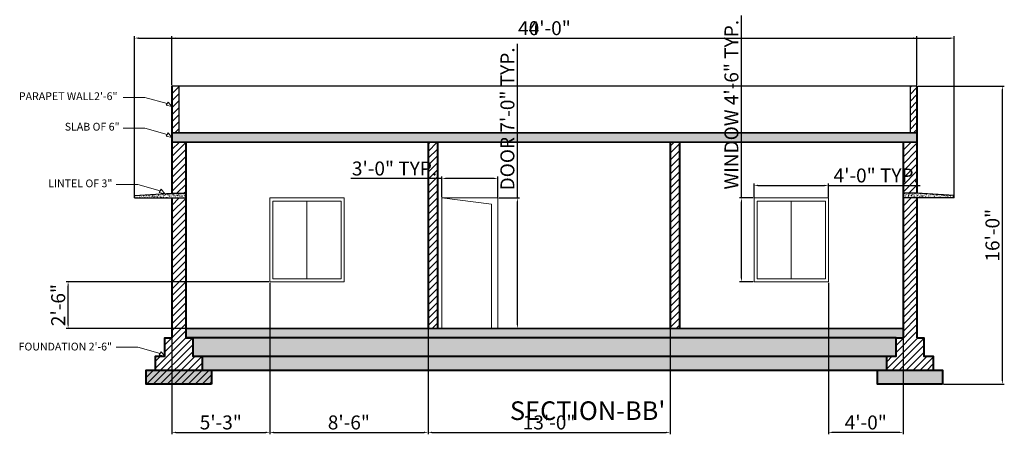
# Model space of a CAD drawing. Units: inches. Extents: x 2639 to 6021, y 292 to 2009.
# Tile 2 of 6: x 3381 to 4016, y 704 to 971. Entities that reach past the tile are written whole.
import ezdxf

# ---------------------------------------------------------------- set-up
doc = ezdxf.new("R2010")
doc.units = ezdxf.units.IN
for name, color, linetype, lineweight in [('A-ANNO-DIMS', 2, 'Continuous', 18), ('A-ANNO-TEXT', 7, 'Continuous', 18), ('A-DOOR', 3, 'Continuous', 20), ('A-GLAZ', 4, 'Continuous', 18), ('A-ROOF', 7, 'Continuous', 30), ('A-SECT', 7, 'Continuous', 40), ('A-SECT-PATT', 8, 'Continuous', 13), ('S-BEAM', 7, 'Continuous', 30), ('S-FNDN', 7, 'Continuous', 40), ('S-SLAB', 7, 'Continuous', 35)]:
    doc.layers.add(name, color=color, linetype=linetype, lineweight=lineweight)
doc.styles.get("Standard").update_dxf_attribs({"font": 'arial.ttf'})
doc.dimstyles.new('ISO-25', dxfattribs={"dimtxt": 9, "dimasz": 2.5, "dimexe": 1.25, "dimexo": 0.625, "dimtad": 1, "dimdec": 1, "dimlunit": 3, "dimtxsty": 'Standard', "dimcen": 2.5, "dimadec": 0, "dimazin": 0, "dimtfac": 1, "dimtdec": 1, "dimtmove": 0, "dimatfit": 3, "dimfxl": 1, "dimarcsym": 0})
pattern_1 = [(50, (-223.561, 0), (18.218467, -1.59391), [1.905, -20.955]), (355, (-223.561, 0), (-3.52434, 19.105685), [1.524, -16.76406]), (100.45144, (-222.043, -0.133), (14.694125, 17.511775), [1.619, -17.809024]), (46.1842, (-223.56, 5.08), (27.1079, -4.20423), [2.8575, -31.4325]), (96.63556, (-221.302, 4.73), (23.74041, 24.74261), [2.4285, -26.71356]), (351.18415, (-223.56, 5.08), (23.74041, 24.74261), [2.286, -25.14597]), (21, (-221.021, 3.81), (15.16144, -10.22652), [1.905, -20.955]), (326, (-221.021, 3.81), (6.1802, 18.4188), [1.524, -16.764]), (71.45144, (-219.758, 2.958), (21.34164, 8.19228), [1.619, -17.80899]), (37.5, (-223.561, 0), (0.30886, 8.455504), [0, -16.5608, 0, -17.018, 0, -16.8275]), (7.5, (-223.561, 0), (6.681966, 10.018057), [0, -9.7028, 0, -16.1798, 0, -6.4135]), (327.5, (-229.225, 0), (13.55906, -0.572874), [0, -6.35, 0, -19.812, 0, -26.289]), (317.5, (-231.765, 0), (14.812918, 2.54265), [0, -8.255, 0, -13.1572, 0, -18.669])]
pattern_2 = [(50, (-223.561, 0), (1.8218467, -0.15939086), [0.1905, -2.0955]), (355, (-223.561, 0), (-0.3524342, 1.91056845), [0.1524, -1.67640584]), (100.451445, (-223.4092, -0.0133), (1.4694125, 1.7511775), [0.1619001, -1.78090245]), (46.1842, (-223.561, 0.508), (2.7107904, -0.4204233), [0.28575, -3.14325]), (96.63556, (-223.3352, 0.473), (2.3740413, 2.4742612), [0.2428502, -2.671356]), (351.18415, (-223.561, 0.508), (2.3740413, 2.4742612), [0.2285997, -2.5145973]), (21, (-223.307, 0.381), (1.5161439, -1.022652), [0.1905, -2.0955]), (326, (-223.307, 0.381), (0.6180203, 1.8418797), [0.1524, -1.6764]), (71.451445, (-223.1807, 0.2958), (2.1341642, 0.8192277), [0.1619001, -1.7808994]), (37.5, (-223.56106, 0), (0.03088603, 0.84555039), [0, -1.65608, 0, -1.7018, 0, -1.68275]), (7.5, (-223.5611, 0), (0.66819663, 1.00180575), [0, -0.97028, 0, -1.61798, 0, -0.64135]), (327.5, (-224.1275, 0), (1.35590595, -0.05728744), [0, -0.635, 0, -1.9812, 0, -2.6289]), (317.5, (-224.3815, 0), (1.4812918, 0.2542649), [0, -0.8255, 0, -1.31572, 0, -1.8669])]

# ---------------------------------------------------------------- blocks, each defined once
blk = doc.blocks.new('DOOR-SECTION-36X84')
for p, q in [((0, 0), (0, 84)), ((0, 84), (36, 84)), ((4, 80), (36, 84)), ((36, 0), (36, 84)), ((4, 0), (4, 80))]:
    blk.add_line(p, q)
blk = doc.blocks.new('WINDOW-SECTION-48X54')
for p, q in [((0, 54), (0, 0)), ((48, 54), (0, 54)), ((2, 52), (2, 2)), ((46, 52), (2, 52)), ((24, 52), (24, 2)), ((46, 52), (46, 2)), ((48, 54), (48, 0)), ((46, 2), (2, 2)), ((48, 0), (0, 0))]:
    blk.add_line(p, q)
blk = doc.blocks.new('NOTE-LEADER-SHORT')
blk.add_lwpolyline([(0, 5.93), (13.88, 5.93), (28.37, 1.9)])
blk.add_lwpolyline([(29.01, 2.92), (27.73, 0.89), (31.32, 0)], close=True)
blk = doc.blocks.new('LINTEL-SECTION-33IN')
for p, q in [((0, 1.5), (24, 3)), ((0, 0), (0, 1.5)), ((24, 3), (33, 3)), ((0, 0), (33, 0))]:
    blk.add_line(p, q)
blk = doc.blocks.new('*D46')
at = {"layer": 'A-ANNO-DIMS', "color": 0, "lineweight": -2, "transparency": 16777216}
for p, q in [((3702.12, 856.63), (3702.12, 956)), ((3690.15, 856.63), (3703.37, 856.63)), ((3702.12, 775.13), (3702.12, 854.13)), ((3690.15, 772.63), (3703.37, 772.63))]:
    blk.add_line(p, q, dxfattribs=at)
at = {"layer": 'A-ANNO-DIMS', "color": 0, "transparency": 16777216}
for points in [[(3701.71, 854.13), (3702.54, 854.13), (3702.12, 856.63)], [(3701.71, 775.13), (3702.54, 775.13), (3702.12, 772.63)]]:
    blk.add_solid(points, dxfattribs=at)
at = {"layer": 'Defpoints', "color": 0, "transparency": 16777216}
for p in [(3689.52, 856.63), (3702.12, 856.63), (3689.52, 772.63)]:
    blk.add_point(p, dxfattribs=at)
at = {"layer": 'A-ANNO-DIMS', "color": 0, "transparency": 16777216, "insert": (3696.84, 907.57), "char_height": 9, "attachment_point": 5, "rotation": 90}
blk.add_mtext('DOOR 7\'-0" TYP.', dxfattribs=at)
blk = doc.blocks.new('*D47')
at = {"layer": 'A-ANNO-DIMS', "color": 0, "lineweight": -2, "transparency": 16777216}
for p, q in [((3653.52, 869.23), (3594.92, 869.23)), ((3653.52, 857.25), (3653.52, 870.48)), ((3687.02, 869.23), (3656.02, 869.23)), ((3689.52, 857.25), (3689.52, 870.48))]:
    blk.add_line(p, q, dxfattribs=at)
at = {"layer": 'A-ANNO-DIMS', "color": 0, "transparency": 16777216}
for points in [[(3656.02, 869.65), (3656.02, 868.81), (3653.52, 869.23)], [(3687.02, 869.65), (3687.02, 868.81), (3689.52, 869.23)]]:
    blk.add_solid(points, dxfattribs=at)
at = {"layer": 'Defpoints', "color": 0, "transparency": 16777216}
for p in [(3653.52, 869.23), (3653.52, 856.63), (3689.52, 856.63)]:
    blk.add_point(p, dxfattribs=at)
at = {"layer": 'A-ANNO-DIMS', "color": 0, "transparency": 16777216, "insert": (3622.97, 874.45), "char_height": 9, "attachment_point": 5}
blk.add_mtext('3\'-0" TYP.', dxfattribs=at)
blk = doc.blocks.new('*D48')
at = {"layer": 'A-ANNO-DIMS', "color": 0, "lineweight": -2, "transparency": 16777216}
for p, q in [((3846.44, 856.63), (3846.44, 974.27)), ((3853.91, 856.63), (3845.19, 856.63)), ((3846.44, 805.13), (3846.44, 854.13)), ((3853.91, 802.63), (3845.19, 802.63))]:
    blk.add_line(p, q, dxfattribs=at)
at = {"layer": 'A-ANNO-DIMS', "color": 0, "transparency": 16777216}
for points in [[(3846.02, 854.13), (3846.85, 854.13), (3846.44, 856.63)], [(3846.02, 805.13), (3846.85, 805.13), (3846.44, 802.63)]]:
    blk.add_solid(points, dxfattribs=at)
at = {"layer": 'Defpoints', "color": 0, "transparency": 16777216}
for p in [(3846.44, 856.63), (3854.54, 856.63), (3854.54, 802.63)]:
    blk.add_point(p, dxfattribs=at)
at = {"layer": 'A-ANNO-DIMS', "color": 0, "transparency": 16777216, "insert": (3841.15, 916.7), "char_height": 9, "attachment_point": 5, "rotation": 90}
blk.add_mtext('WINDOW 4\'-6" TYP.', dxfattribs=at)
blk = doc.blocks.new('*D49')
at = {"layer": 'A-ANNO-DIMS', "color": 0, "lineweight": -2, "transparency": 16777216}
for p, q in [((3854.54, 857.25), (3854.54, 865.98)), ((3857.04, 864.73), (3900.04, 864.73)), ((3902.54, 857.25), (3902.54, 865.98)), ((3902.54, 864.73), (3961.51, 864.73))]:
    blk.add_line(p, q, dxfattribs=at)
at = {"layer": 'A-ANNO-DIMS', "color": 0, "transparency": 16777216}
for points in [[(3857.04, 865.15), (3857.04, 864.31), (3854.54, 864.73)], [(3900.04, 865.15), (3900.04, 864.31), (3902.54, 864.73)]]:
    blk.add_solid(points, dxfattribs=at)
at = {"layer": 'Defpoints', "color": 0, "transparency": 16777216}
for p in [(3902.54, 864.73), (3854.54, 856.63), (3902.54, 856.63)]:
    blk.add_point(p, dxfattribs=at)
at = {"layer": 'A-ANNO-DIMS', "color": 0, "transparency": 16777216, "insert": (3933.27, 869.95), "char_height": 9, "attachment_point": 5}
blk.add_mtext('4\'-0" TYP.', dxfattribs=at)
blk = doc.blocks.new('*D104')
at = {"layer": 'A-ANNO-DIMS', "color": 0, "lineweight": -2, "transparency": 16777216}
for p, q in [((3455.54, 857.25), (3455.54, 960.88)), ((3458.04, 959.63), (3981.04, 959.63)), ((3983.54, 857.25), (3983.54, 960.88))]:
    blk.add_line(p, q, dxfattribs=at)
at = {"layer": 'A-ANNO-DIMS', "color": 0, "transparency": 16777216}
for points in [[(3458.04, 960.05), (3458.04, 959.21), (3455.54, 959.63)], [(3981.04, 960.05), (3981.04, 959.21), (3983.54, 959.63)]]:
    blk.add_solid(points, dxfattribs=at)
at = {"layer": 'Defpoints', "color": 0, "transparency": 16777216}
for p in [(3983.54, 959.63), (3455.54, 856.63), (3983.54, 856.63)]:
    blk.add_point(p, dxfattribs=at)
at = {"layer": 'A-ANNO-DIMS', "color": 0, "transparency": 16777216, "insert": (3719.54, 964.85), "char_height": 9, "attachment_point": 5}
blk.add_mtext('44\'-0"', dxfattribs=at)
blk = doc.blocks.new('*D105')
at = {"layer": 'A-ANNO-DIMS', "color": 0, "lineweight": -2, "transparency": 16777216}
for p, q in [((3479.54, 929.25), (3479.54, 960.88)), ((3482.04, 959.63), (3957.04, 959.63)), ((3959.54, 929.25), (3959.54, 960.88))]:
    blk.add_line(p, q, dxfattribs=at)
at = {"layer": 'A-ANNO-DIMS', "color": 0, "transparency": 16777216}
for points in [[(3482.04, 960.05), (3482.04, 959.21), (3479.54, 959.63)], [(3957.04, 960.05), (3957.04, 959.21), (3959.54, 959.63)]]:
    blk.add_solid(points, dxfattribs=at)
at = {"layer": 'Defpoints', "color": 0, "transparency": 16777216}
for p in [(3959.54, 959.63), (3479.54, 928.63), (3959.54, 928.63)]:
    blk.add_point(p, dxfattribs=at)
at = {"layer": 'A-ANNO-DIMS', "color": 0, "transparency": 16777216, "insert": (3719.54, 964.85), "char_height": 9, "attachment_point": 5}
blk.add_mtext('40\'-0"', dxfattribs=at)
blk = doc.blocks.new('*D106')
at = {"layer": 'A-ANNO-DIMS', "color": 0, "lineweight": -2, "transparency": 16777216}
for p, q in [((3960.16, 928.63), (4015.79, 928.63)), ((4014.54, 739.13), (4014.54, 926.13)), ((3976.66, 736.63), (4015.79, 736.63))]:
    blk.add_line(p, q, dxfattribs=at)
at = {"layer": 'A-ANNO-DIMS', "color": 0, "transparency": 16777216}
for points in [[(4014.12, 926.13), (4014.95, 926.13), (4014.54, 928.63)], [(4014.12, 739.13), (4014.95, 739.13), (4014.54, 736.63)]]:
    blk.add_solid(points, dxfattribs=at)
at = {"layer": 'Defpoints', "color": 0, "transparency": 16777216}
for p in [(3959.54, 928.63), (4014.54, 928.63), (3976.04, 736.63)]:
    blk.add_point(p, dxfattribs=at)
at = {"layer": 'A-ANNO-DIMS', "color": 0, "transparency": 16777216, "insert": (4009.32, 832.63), "char_height": 9, "attachment_point": 5, "rotation": 90}
blk.add_mtext('16\'-0"', dxfattribs=at)
blk = doc.blocks.new('*D107')
at = {"layer": 'A-ANNO-DIMS', "color": 0, "lineweight": -2, "transparency": 16777216}
for p, q in [((3542.54, 802), (3542.54, 704.38)), ((3479.54, 766), (3479.54, 704.38)), ((3482.04, 705.63), (3540.04, 705.63))]:
    blk.add_line(p, q, dxfattribs=at)
at = {"layer": 'A-ANNO-DIMS', "color": 0, "transparency": 16777216}
for points in [[(3482.04, 706.05), (3482.04, 705.21), (3479.54, 705.63)], [(3540.04, 706.05), (3540.04, 705.21), (3542.54, 705.63)]]:
    blk.add_solid(points, dxfattribs=at)
at = {"layer": 'Defpoints', "color": 0, "transparency": 16777216}
for p in [(3542.54, 802.63), (3479.54, 766.63), (3542.54, 705.63)]:
    blk.add_point(p, dxfattribs=at)
at = {"layer": 'A-ANNO-DIMS', "color": 0, "transparency": 16777216, "insert": (3511.04, 710.85), "char_height": 9, "attachment_point": 5}
blk.add_mtext('5\'-3"', dxfattribs=at)
blk = doc.blocks.new('*D108')
at = {"layer": 'A-ANNO-DIMS', "color": 0, "lineweight": -2, "transparency": 16777216}
for p, q in [((3542.54, 802), (3542.54, 704.38)), ((3644.54, 772), (3644.54, 704.38)), ((3545.04, 705.63), (3642.04, 705.63))]:
    blk.add_line(p, q, dxfattribs=at)
at = {"layer": 'A-ANNO-DIMS', "color": 0, "transparency": 16777216}
for points in [[(3545.04, 706.05), (3545.04, 705.21), (3542.54, 705.63)], [(3642.04, 706.05), (3642.04, 705.21), (3644.54, 705.63)]]:
    blk.add_solid(points, dxfattribs=at)
at = {"layer": 'Defpoints', "color": 0, "transparency": 16777216}
for p in [(3542.54, 802.63), (3644.54, 772.63), (3644.54, 705.63)]:
    blk.add_point(p, dxfattribs=at)
at = {"layer": 'A-ANNO-DIMS', "color": 0, "transparency": 16777216, "insert": (3593.54, 710.85), "char_height": 9, "attachment_point": 5}
blk.add_mtext('8\'-6"', dxfattribs=at)
blk = doc.blocks.new('*D109')
at = {"layer": 'A-ANNO-DIMS', "color": 0, "lineweight": -2, "transparency": 16777216}
for p, q in [((3644.54, 772), (3644.54, 704.38)), ((3800.54, 772), (3800.54, 704.38)), ((3647.04, 705.63), (3798.04, 705.63))]:
    blk.add_line(p, q, dxfattribs=at)
at = {"layer": 'A-ANNO-DIMS', "color": 0, "transparency": 16777216}
for points in [[(3647.04, 706.05), (3647.04, 705.21), (3644.54, 705.63)], [(3798.04, 706.05), (3798.04, 705.21), (3800.54, 705.63)]]:
    blk.add_solid(points, dxfattribs=at)
at = {"layer": 'Defpoints', "color": 0, "transparency": 16777216}
for p in [(3644.54, 772.63), (3800.54, 772.63), (3800.54, 705.63)]:
    blk.add_point(p, dxfattribs=at)
at = {"layer": 'A-ANNO-DIMS', "color": 0, "transparency": 16777216, "insert": (3722.54, 710.85), "char_height": 9, "attachment_point": 5}
blk.add_mtext('13\'-0"', dxfattribs=at)
blk = doc.blocks.new('*D110')
at = {"layer": 'A-ANNO-DIMS', "color": 0, "lineweight": -2, "transparency": 16777216}
for p, q in [((3902.54, 802), (3902.54, 704.38)), ((3950.54, 772), (3950.54, 704.38)), ((3948.04, 705.63), (3905.04, 705.63))]:
    blk.add_line(p, q, dxfattribs=at)
at = {"layer": 'A-ANNO-DIMS', "color": 0, "transparency": 16777216}
for points in [[(3905.04, 706.05), (3905.04, 705.21), (3902.54, 705.63)], [(3948.04, 706.05), (3948.04, 705.21), (3950.54, 705.63)]]:
    blk.add_solid(points, dxfattribs=at)
at = {"layer": 'Defpoints', "color": 0, "transparency": 16777216}
for p in [(3902.54, 802.63), (3950.54, 772.63), (3902.54, 705.63)]:
    blk.add_point(p, dxfattribs=at)
at = {"layer": 'A-ANNO-DIMS', "color": 0, "transparency": 16777216, "insert": (3926.54, 710.85), "char_height": 9, "attachment_point": 5}
blk.add_mtext('4\'-0"', dxfattribs=at)
blk = doc.blocks.new('*D111')
at = {"layer": 'A-ANNO-DIMS', "color": 0, "lineweight": -2, "transparency": 16777216}
for p, q in [((3541.91, 802.63), (3411.43, 802.63)), ((3412.68, 775.13), (3412.68, 800.13)), ((3487.91, 772.63), (3411.43, 772.63))]:
    blk.add_line(p, q, dxfattribs=at)
at = {"layer": 'A-ANNO-DIMS', "color": 0, "transparency": 16777216}
for points in [[(3412.27, 800.13), (3413.1, 800.13), (3412.68, 802.63)], [(3412.27, 775.13), (3413.1, 775.13), (3412.68, 772.63)]]:
    blk.add_solid(points, dxfattribs=at)
at = {"layer": 'Defpoints', "color": 0, "transparency": 16777216}
for p in [(3412.68, 802.63), (3542.54, 802.63), (3488.54, 772.63)]:
    blk.add_point(p, dxfattribs=at)
at = {"layer": 'A-ANNO-DIMS', "color": 0, "transparency": 16777216, "insert": (3407.46, 787.63), "char_height": 9, "attachment_point": 5, "rotation": 90}
blk.add_mtext('2\'-6"', dxfattribs=at)

msp = doc.modelspace()

# ---------------------------------------------------------------- hatches: boundary and pattern name
at = {"layer": 'A-SECT-PATT'}
h = msp.add_hatch(dxfattribs=at)
h.set_pattern_fill('ANSI31', color=256)
h.set_pattern_definition([(45, (-223.561, 0), (-2.245064, 2.245064), [])])
h.paths.add_polyline_path([(3484.04, 928.63), (3479.54, 928.63), (3479.54, 898.63), (3484.04, 898.63)])
h.paths.add_polyline_path([(3488.54, 856.63), (3479.54, 856.63), (3479.54, 766.63), (3475.04, 766.63), (3475.04, 754.63), (3469.04, 754.63), (3469.04, 745.63), (3463.04, 745.63), (3463.04, 736.63), (3505.04, 736.63), (3505.04, 745.63), (3499.04, 745.63), (3499.04, 754.63), (3493.04, 754.63), (3493.04, 766.63), (3488.54, 766.63)])
h.paths.add_polyline_path([(3488.54, 892.63), (3479.54, 892.63), (3479.54, 859.63), (3488.54, 859.63)])
h.paths.add_polyline_path([(3650.54, 892.63), (3644.54, 892.63), (3644.54, 772.63), (3650.54, 772.63)])
h.paths.add_polyline_path([(3806.54, 892.63), (3800.54, 892.63), (3800.54, 772.63), (3806.54, 772.63)])
h.paths.add_polyline_path([(3959.54, 892.63), (3950.54, 892.63), (3950.54, 859.63), (3959.54, 859.63)])
h.paths.add_polyline_path([(3959.54, 856.63), (3950.54, 856.63), (3950.54, 766.63), (3946.04, 766.63), (3946.04, 754.63), (3940.04, 754.63), (3940.04, 745.63), (3970.04, 745.63), (3970.04, 754.63), (3964.04, 754.63), (3964.04, 766.63), (3959.54, 766.63)])
h.paths.add_polyline_path([(3959.54, 928.63), (3955.04, 928.63), (3955.04, 898.63), (3959.54, 898.63)])
h = msp.add_hatch(dxfattribs=at)
h.set_pattern_fill('AR-CONC', color=256, scale=0.1)
h.set_pattern_definition(pattern_1)
h.paths.add_polyline_path([(3479.54, 898.63), (3479.54, 892.63), (3959.54, 892.63), (3959.54, 898.63)])
h = msp.add_hatch(dxfattribs=at)
h.set_pattern_fill('AR-CONC', color=256, scale=0.01)
h.set_pattern_definition(pattern_2)
h.paths.add_polyline_path([(3488.54, 859.63), (3479.54, 859.63), (3455.54, 858.13), (3455.54, 856.63), (3488.54, 856.63)])
h = msp.add_hatch(dxfattribs=at)
h.set_pattern_fill('AR-CONC', color=256, scale=0.01)
h.set_pattern_definition(pattern_2)
h.paths.add_polyline_path([(3983.54, 858.13), (3959.54, 859.63), (3950.54, 859.63), (3950.54, 856.63), (3983.54, 856.63)])
h = msp.add_hatch(dxfattribs=at)
h.set_pattern_fill('AR-SAND', color=256, scale=0.1)
h.set_pattern_definition([(37.5, (-223.561, 0), (-0.160003, 4.8941324), [0, -3.8608, 0, -4.318, 0, -4.1275]), (7.5, (-223.561, 0), (4.495233, 7.168251), [0, -2.0828, 0, -3.4798, 0, -1.3335]), (327.5, (-226.6853, 0), (7.9099237, 0.014372), [0, -1.27, 0, -4.572, 0, -5.969]), (317.5, (-226.685, 0), (7.635565, 2.229293), [0, -0.635, 0, -2.9972, 0, -3.429])])
h.paths.add_polyline_path([(3946.05, 766.63), (3950.54, 766.63), (3950.54, 772.63), (3488.54, 772.63), (3488.54, 766.63), (3493.04, 766.63)])
h = msp.add_hatch(dxfattribs=at)
h.set_pattern_fill('AR-CONC', color=256, scale=0.1)
h.set_pattern_definition(pattern_1)
h.paths.add_polyline_path([(3493.04, 766.63), (3493.04, 754.63), (3499.04, 754.63), (3940.04, 754.63), (3946.04, 754.63), (3946.04, 766.63)])
h = msp.add_hatch(dxfattribs=at)
h.set_pattern_fill('GRAVEL', color=256, scale=0.5)
h.set_pattern_definition([(228.012788, (-214.4171, 12.7), (-101.6, -114.3), [1.708607, -169.15242]), (184.969741, (-215.56006, 11.43), (152.39999994, 12.70000072), [2.932024, -290.270244]), (132.510447, (-218.48106, 11.176), (127.00000005, -139.69999995), [2.067408, -204.673614]), (267.273689, (-223.43406, 8.001), (12.70000003, 254), [2.670023, -264.332187]), (292.833654, (-223.56106, 5.334), (-63.500000005, 152.4), [2.61817, -259.19904]), (357.273689, (-222.54506, 2.921), (-254, 12.70000003), [2.670023, -264.332187]), (37.69424, (-219.87806, 2.794), (-165.099999993, -127.00000001), [3.53097, -349.565577]), (72.255328, (-217.08406, 4.953), (88.900000024, 279.39999999), [3.333598, -330.026283]), (121.429566, (-216.06806, 8.128), (-101.600000014, 165.09999999), [2.679065, -265.22773]), (175.236358, (-217.4651, 10.414), (139.7, -12.70000002), [3.058566, -149.869685]), (222.397438, (-220.51306, 10.668), (-152.399999995, -139.700000005), [3.95539, -391.583863]), (138.814075, (-210.861, 7.874), (-88.9, 76.2), [1.350023, -133.65283]), (171.469234, (-211.87706, 8.763), (165.1, -25.39999997), [2.56841, -254.273195]), (225, (-214.417, 9.144), (-2e-15, -12.7), [1.796047, -16.164466]), (203.19859, (-215.306, 10.668), (63.5, 25.4), [0.967207, -95.75311]), (291.80141, (-216.195, 10.287), (-12.7, 38.1), [1.367828, -67.023765]), (30.963757, (-215.687, 9.017), (38.1, 25.4), [2.2216, -71.83149]), (161.56505, (-213.782, 10.16), (25.4, -12.7), [1.606436, -38.55449]), (16.38954, (-223.56106, 10.287), (127, 38.1), [2.25044, -222.794133]), (70.346176, (-221.40206, 10.922), (-50.8, -139.7), [1.887995, -186.91108]), (293.19859, (-213.782, 12.7), (-25.4, 63.5), [1.9344, -94.785918]), (343.61046, (-213.02006, 10.922), (-127, 38.09999999), [2.25044, -222.794133]), (339.443955, (-223.561, 2.413), (-63.5, 25.4), [2.170176, -106.33867]), (294.77514, (-221.5291, 1.651), (-63.50000008, 139.69999997), [1.81836, -180.017967]), (66.80141, (-213.655, 0), (25.4, 63.5), [1.9344, -94.785918]), (17.354025, (-212.89306, 1.778), (-165.1, -50.80000001), [2.128914, -210.76188]), (69.443955, (-219.878, 0), (-25.4, -63.5), [1.085088, -107.42376]), (101.30993, (-214.417, 0), (-12.7, 50.8), [0.647573, -64.109975]), (165.96376, (-214.544, 0.635), (38.1, -12.7), [2.61817, -49.745273]), (186.009006, (-217.08406, 1.27), (127, 12.70000001), [2.426335, -240.206824]), (303.69007, (-215.687, 7.874), (-12.7, 25.4), [1.83162, -43.95888]), (353.157227, (-214.67106, 6.35), (215.9, -25.39999999), [3.197784, -316.580045]), (60.945396, (-211.496, 5.969), (-50.8, -88.9), [1.30754, -129.44696]), (90, (-210.861, 7.112), (-12.7, 12.7), [0.762, -11.938]), (120.256437, (-217.3381, 1.651), (50.8, -88.9), [1.764335, -174.669704]), (48.012787, (-218.2271, 3.175), (101.6, 114.3), [3.417214, -167.44381]), (0, (-215.941, 5.715), (12.7, 12.7), [3.302, -9.398]), (325.304846, (-212.63906, 5.715), (127.00000005, -88.89999993), [2.008048, -198.796584]), (254.054604, (-210.988, 4.572), (-12.7, -50.8), [1.849145, -90.60825]), (207.645975, (-211.49606, 2.794), (-241.30000001, -126.99999998), [3.010725, -298.062322]), (175.426079, (-214.16306, 1.397), (-165.1, 12.7), [3.185147, -315.329232])])
h.paths.add_polyline_path([(3499.04, 754.63), (3499.04, 745.63), (3505.04, 745.63), (3934.04, 745.63), (3940.04, 745.63), (3940.04, 754.63)])
h = msp.add_hatch(dxfattribs=at)
h.set_pattern_fill('AR-CONC', color=256, scale=0.1)
h.set_pattern_definition(pattern_1)
h.paths.add_polyline_path([(3505.04, 736.63), (3505.04, 745.63), (3499.04, 745.63), (3469.04, 745.63), (3463.04, 745.63), (3463.04, 736.63)])
h.paths.add_polyline_path([(3976.04, 736.63), (3976.04, 745.63), (3970.04, 745.63), (3940.04, 745.63), (3934.04, 745.63), (3934.04, 736.63)])

# ---------------------------------------------------------------- linework, layer by layer
at = {"layer": 'A-ROOF'}
for p, q in [((3959.54, 928.63), (3479.54, 928.63)), ((3484.04, 928.63), (3484.04, 898.63)), ((3955.04, 928.63), (3955.04, 898.63))]:
    msp.add_line(p, q, dxfattribs=at)
at = {"layer": 'A-SECT'}
for p, q in [((3479.54, 928.63), (3479.54, 859.63)), ((3959.54, 928.63), (3959.54, 859.63)), ((3488.54, 892.63), (3488.54, 766.63)), ((3644.54, 892.63), (3644.54, 772.63)), ((3650.54, 892.63), (3650.54, 772.63)), ((3800.54, 892.63), (3800.54, 772.63)), ((3806.54, 892.63), (3806.54, 772.63)), ((3950.54, 892.63), (3950.54, 766.63)), ((3479.54, 856.63), (3479.54, 766.63)), ((3959.54, 856.63), (3959.54, 766.63))]:
    msp.add_line(p, q, dxfattribs=at)
at = {"layer": 'S-FNDN'}
for p, q in [((3946.05, 766.63), (3488.54, 766.63)), ((3499.04, 754.63), (3940.04, 754.63)), ((3469.04, 745.63), (3499.04, 745.63)), ((3505.04, 745.63), (3934.04, 745.63)), ((3940.04, 745.63), (3970.04, 745.63))]:
    msp.add_line(p, q, dxfattribs=at)
for points in [[(3505.04, 736.63), (3463.04, 736.63), (3463.04, 745.63), (3469.04, 745.63), (3469.04, 754.63), (3475.04, 754.63), (3475.04, 766.63), (3479.54, 766.63)], [(3488.54, 766.63), (3493.04, 766.63), (3493.04, 754.63), (3499.04, 754.63), (3499.04, 745.63), (3505.04, 745.63), (3505.04, 736.63)], [(3976.04, 736.63), (3934.04, 736.63), (3934.04, 745.63), (3940.04, 745.63), (3940.04, 754.63), (3946.04, 754.63), (3946.04, 766.63), (3950.54, 766.63)], [(3959.54, 766.63), (3964.04, 766.63), (3964.04, 754.63), (3970.04, 754.63), (3970.04, 745.63), (3976.04, 745.63), (3976.04, 736.63)]]:
    msp.add_lwpolyline(points, dxfattribs=at)
at = {"layer": 'S-SLAB'}
for p, q in [((3959.54, 898.63), (3479.54, 898.63)), ((3959.54, 892.63), (3479.54, 892.63)), ((3950.54, 772.63), (3488.54, 772.63))]:
    msp.add_line(p, q, dxfattribs=at)

# ---------------------------------------------------------------- block references
at = {"layer": 'A-ANNO-TEXT'}
for p in [(3448.21, 915.51), (3448.21, 895.64), (3443.68, 859.35), (3443.71, 754.63)]:
    msp.add_blockref('NOTE-LEADER-SHORT', p, dxfattribs=at)
at = {"layer": 'A-DOOR', "extrusion": (0, 0, -1), "zscale": -1}
msp.add_blockref('DOOR-SECTION-36X84', (-3689.52, 772.63), dxfattribs=at)
at = {"layer": 'A-GLAZ', "rotation": 180}
msp.add_blockref('WINDOW-SECTION-48X54', (3590.54, 856.63), dxfattribs=at)
at = {"layer": 'A-GLAZ'}
msp.add_blockref('WINDOW-SECTION-48X54', (3854.54, 802.63), dxfattribs=at)
at = {"layer": 'S-BEAM'}
msp.add_blockref('LINTEL-SECTION-33IN', (3455.54, 856.63), dxfattribs=at)
at = {"layer": 'S-BEAM', "extrusion": (0, 0, -1), "zscale": -1}
msp.add_blockref('LINTEL-SECTION-33IN', (-3983.54, 856.63), dxfattribs=at)

# ---------------------------------------------------------------- texts
at = {"layer": 'A-ANNO-TEXT', "attachment_point": 1}
for s, width, heights, insert, char_height in [('{\\fTimes New Roman|b0|i0|c0|p18;PARAPET WALL2\'-6"}', 172.2916, [0], (3380.99, 924.7), 5), ('{\\fTimes New Roman|b0|i0|c0|p18;SLAB OF 6"}', 40.7521, [5.11], (3410.53, 905.04), 5), ('{\\fTimes New Roman|b0|i0|c0|p18;LINTEL OF 3"}', 49.0691, [0], (3399.87, 868.53), 5), ('{\\fTimes New Roman|b0|i0|c0|p18;FOUNDATION 2\'-6"}', 65.4654, [0], (3380.8, 763.39), 5), ("{\\fTimes New Roman|b0|i0|c0|p18;SECTION-BB'}", 172.2916, [0], (3697.3, 725.6), 12)]:
    msp.add_mtext_dynamic_manual_height_columns(s, width=width, gutter_width=12.5, heights=heights, dxfattribs=dict(at, insert=insert, char_height=char_height))

# ---------------------------------------------------------------- dimensions: what is measured, and where the dimension line sits
at = {"layer": 'A-ANNO-DIMS'}
for base, p1, p2, picture, middle in [((3983.54, 959.63), (3455.54, 856.63), (3983.54, 856.63), '*D104', (3719.54, 964.85)), ((3959.54, 959.63), (3479.54, 928.63), (3959.54, 928.63), '*D105', (3719.54, 964.85)), ((3542.54, 705.63), (3479.54, 766.63), (3542.54, 802.63), '*D107', (3511.04, 710.85)), ((3644.54, 705.63), (3542.54, 802.63), (3644.54, 772.63), '*D108', (3593.54, 710.85)), ((3902.54, 705.63), (3950.54, 772.63), (3902.54, 802.63), '*D110', (3926.54, 710.85)), ((3800.54, 705.63), (3644.54, 772.63), (3800.54, 772.63), '*D109', (3722.54, 710.85))]:
    dim = msp.add_linear_dim(base=base, p1=p1, p2=p2, dimstyle='ISO-25', override={"dimdec": 1, "dimlfac": 1, "dimrnd": 0, "dimzin": 1, "dimdsep": 46, "dimlunit": 4, "dimfrac": 2}, dxfattribs=at)
    dim.commit()
    dim.dimension.update_dxf_attribs({"geometry": picture, "text_midpoint": middle})
for base, p1, p2, angle, text, picture, middle in [((3846.44, 856.63), (3854.54, 802.63), (3854.54, 856.63), 90, 'WINDOW <> TYP.', '*D48', (3841.15, 916.7)), ((3702.12, 856.63), (3689.52, 772.63), (3689.52, 856.63), 90, 'DOOR <> TYP.', '*D46', (3696.84, 907.57)), ((3653.52, 869.23), (3689.52, 856.63), (3653.52, 856.63), 180, '<> TYP.', '*D47', (3622.97, 874.45))]:
    dim = msp.add_linear_dim(base=base, p1=p1, p2=p2, angle=angle, text=text, dimstyle='ISO-25', override={"dimdec": 1, "dimlfac": 1, "dimrnd": 0, "dimzin": 1, "dimdsep": 46, "dimlunit": 4, "dimfrac": 2}, dxfattribs=at)
    dim.commit()
    dim.dimension.update_dxf_attribs({"geometry": picture, "text_midpoint": middle})
for base, p1, p2, picture, middle in [((4014.54, 928.63), (3976.04, 736.63), (3959.54, 928.63), '*D106', (4009.32, 832.63)), ((3412.68, 802.63), (3488.54, 772.63), (3542.54, 802.63), '*D111', (3407.46, 787.63))]:
    dim = msp.add_linear_dim(base=base, p1=p1, p2=p2, angle=90, dimstyle='ISO-25', override={"dimdec": 1, "dimlfac": 1, "dimrnd": 0, "dimzin": 1, "dimdsep": 46, "dimlunit": 4, "dimfrac": 2}, dxfattribs=at)
    dim.commit()
    dim.dimension.update_dxf_attribs({"geometry": picture, "text_midpoint": middle})
dim = msp.add_linear_dim(base=(3902.54, 864.73), p1=(3854.54, 856.63), p2=(3902.54, 856.63), text='<> TYP.', dimstyle='ISO-25', override={"dimdec": 1, "dimlfac": 1, "dimrnd": 0, "dimzin": 1, "dimdsep": 46, "dimlunit": 4, "dimfrac": 2}, dxfattribs=at)
dim.commit()
dim.dimension.update_dxf_attribs({"geometry": '*D49', "text_midpoint": (3933.27, 869.95)})

doc.saveas('drawing.dxf')
